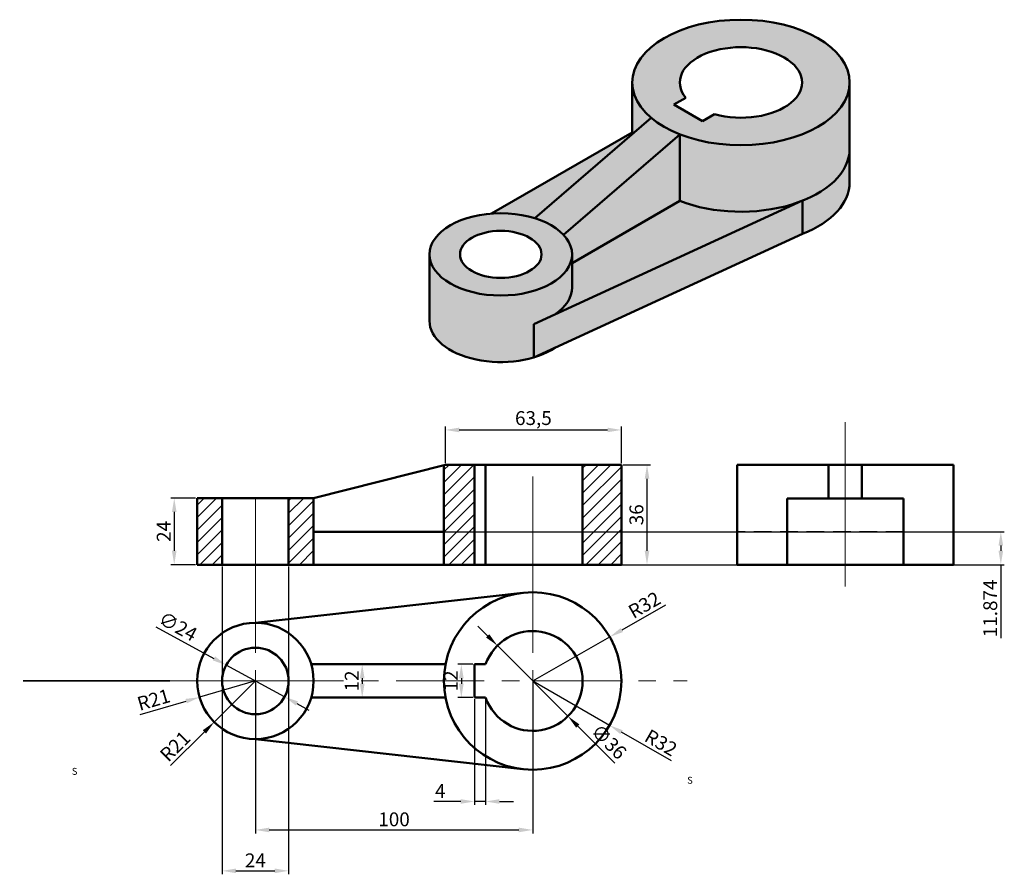
# Model space of a CAD drawing. Units: millimetres. Extents: x -12 to 343, y -126 to 182.
import ezdxf

# ---------------------------------------------------------------- set-up
doc = ezdxf.new("R2010")
doc.units = ezdxf.units.MM
for name, pattern in [('CENTER', [50.800000000000004, 31.75, -6.349999999999999, 6.349999999999999, -6.349999999999999]), ('HIDDEN', [9.524999999999999, 6.349999999999999, -3.174999999999999]), ('PHANTOM', [63.50000000000001, 31.75, -6.349999999999999, 6.349999999999999, -6.349999999999999, 6.349999999999999, -6.349999999999999])]:
    doc.linetypes.add(name, pattern=pattern)
for name, color, linetype, lineweight in [('M-CNTR', 1, 'CENTER', 18), ('M-DIMS', 2, 'Continuous', 25), ('M-HATC', 251, 'Continuous', 18), ('M-HIDN', 4, 'HIDDEN', 25), ('M-OUTL', 7, 'Continuous', 50), ('M-SECT', 6, 'PHANTOM', 35), ('M-TEXT', 3, 'Continuous', 25)]:
    doc.layers.add(name, color=color, linetype=linetype, lineweight=lineweight)
doc.styles.get("Standard").update_dxf_attribs({"font": 'arial.ttf'})
doc.dimstyles.new('ISO-25', dxfattribs={"dimtxt": 5, "dimasz": 5, "dimexe": 1.25, "dimexo": 0.625, "dimtad": 1, "dimtxsty": 'Standard', "dimcen": 5, "dimadec": 0, "dimazin": 0, "dimtfac": 1, "dimtmove": 0, "dimatfit": 3, "dimfxl": 1, "dimarcsym": 0})
pattern_1 = [(45, (0, 0), (-2.245064030267288, 2.245064030267288), [])]

# ---------------------------------------------------------------- blocks, each defined once
blk = doc.blocks.new('*D1')
at = {"layer": 'Defpoints', "color": 0, "transparency": 16777216}
for p in [(205.2649197556575, 34.47405386195669), (141.7649197556575, 21.88545579629272), (205.2649197556575, 21.88545579629272)]:
    blk.add_point(p, dxfattribs=at)
at = {"layer": 'M-DIMS', "color": 0, "lineweight": -2, "transparency": 16777216}
for p, q in [((141.7649197556575, 22.51045579629272), (141.7649197556575, 35.72405386195669)), ((205.2649197556575, 22.51045579629272), (205.2649197556575, 35.72405386195669)), ((146.7649197556575, 34.47405386195669), (200.2649197556575, 34.47405386195669))]:
    blk.add_line(p, q, dxfattribs=at)
at = {"layer": 'M-DIMS', "color": 0, "transparency": 16777216}
for points in [[(146.7649197556575, 35.30738719529003), (146.7649197556575, 33.64072052862336), (141.7649197556575, 34.47405386195669)], [(200.2649197556575, 35.30738719529003), (200.2649197556575, 33.64072052862336), (205.2649197556575, 34.47405386195669)]]:
    blk.add_solid(points, dxfattribs=at)
at = {"layer": 'M-DIMS', "color": 0, "transparency": 16777216, "insert": (173.5149197556575, 38.10382875963745), "char_height": 5, "attachment_point": 5}
blk.add_mtext('63,5', dxfattribs=at)
blk = doc.blocks.new('*D2')
at = {"layer": 'Defpoints', "color": 0, "transparency": 16777216}
for p in [(205.2649197556577, 21.88545579629272), (214.4923014426937, 21.88545579629272), (205.2649197556577, -14.11454420370729)]:
    blk.add_point(p, dxfattribs=at)
at = {"layer": 'M-DIMS', "color": 0, "lineweight": -2, "transparency": 16777216}
for p, q in [((205.8899197556577, 21.88545579629272), (215.7423014426937, 21.88545579629272)), ((214.4923014426937, -9.114544203707284), (214.4923014426937, 16.88545579629272)), ((205.8899197556577, -14.11454420370729), (215.7423014426937, -14.11454420370728))]:
    blk.add_line(p, q, dxfattribs=at)
at = {"layer": 'M-DIMS', "color": 0, "transparency": 16777216}
for points in [[(213.6589681093604, 16.88545579629272), (215.3256347760271, 16.88545579629272), (214.4923014426937, 21.88545579629272)], [(213.6589681093604, -9.114544203707284), (215.3256347760271, -9.114544203707284), (214.4923014426937, -14.11454420370728)]]:
    blk.add_solid(points, dxfattribs=at)
at = {"layer": 'M-DIMS', "color": 0, "transparency": 16777216, "insert": (211.3127311834849, 3.885455796292659), "char_height": 5, "attachment_point": 5, "rotation": 90}
blk.add_mtext('36', dxfattribs=at)
blk = doc.blocks.new('*D3')
at = {"layer": 'Defpoints', "color": 0, "transparency": 16777216}
for p in [(52.26491975565753, 9.88545579629272), (43.9988590508993, -14.11454420370729), (52.26491975565753, -14.11454420370729)]:
    blk.add_point(p, dxfattribs=at)
at = {"layer": 'M-DIMS', "color": 0, "lineweight": -2, "transparency": 16777216}
for p, q in [((51.63991975565753, 9.88545579629272), (42.7488590508993, 9.885455796292717)), ((43.9988590508993, 4.885455796292717), (43.9988590508993, -9.114544203707291)), ((51.63991975565753, -14.11454420370729), (42.7488590508993, -14.11454420370729))]:
    blk.add_line(p, q, dxfattribs=at)
at = {"layer": 'M-DIMS', "color": 0, "transparency": 16777216}
for points in [[(43.16552571756596, 4.885455796292717), (44.83219238423263, 4.885455796292717), (43.9988590508993, 9.885455796292717)], [(43.16552571756596, -9.114544203707291), (44.83219238423263, -9.11454420370729), (43.9988590508993, -14.11454420370729)]]:
    blk.add_solid(points, dxfattribs=at)
at = {"layer": 'M-DIMS', "color": 0, "transparency": 16777216, "insert": (40.86362712729765, -2.114544203707298), "char_height": 5, "attachment_point": 5, "rotation": 90}
blk.add_mtext('24', dxfattribs=at)
blk = doc.blocks.new('*D4')
at = {"layer": 'Defpoints', "color": 0, "transparency": 16777216}
for p in [(73.2649197556575, -56.05038137719969), (53.10428194249988, -61.92819414783812)]:
    blk.add_point(p, dxfattribs=at)
at = {"layer": 'M-DIMS', "color": 0, "lineweight": -2, "transparency": 16777216}
for p, q in [((73.2649197556575, -56.05038137719969), (53.10428194249988, -61.92819414783812)), ((31.76063262380506, -68.15091267986675), (48.30413008222426, -63.3276733789425))]:
    blk.add_line(p, q, dxfattribs=at)
at = {"layer": 'M-DIMS', "color": 0, "transparency": 16777216}
blk.add_solid([(48.07088354370687, -62.52764806889658), (48.53737662074166, -64.12769868898843), (53.10428194249988, -61.92819414783812)], dxfattribs=at)
at = {"layer": 'M-DIMS', "color": 0, "transparency": 16777216, "insert": (36.75476703052166, -63.42911477486243), "char_height": 5, "attachment_point": 5, "rotation": 16.253988585853655}
blk.add_mtext('R21', dxfattribs=at)
blk = doc.blocks.new('*D5')
at = {"layer": 'Defpoints', "color": 0, "transparency": 16777216}
for p in [(201.0521765959829, -40.18002040809157), (173.2649197556575, -56.05038137719977)]:
    blk.add_point(p, dxfattribs=at)
at = {"layer": 'M-DIMS', "color": 0, "lineweight": -2, "transparency": 16777216}
for p, q in [((221.1513216491535, -28.70063296811324), (205.3939354772837, -37.70027650666842)), ((173.2649197556575, -56.05038137719977), (201.0521765959829, -40.18002040809157))]:
    blk.add_line(p, q, dxfattribs=at)
at = {"layer": 'M-DIMS', "color": 0, "transparency": 16777216}
blk.add_solid([(204.9806448270465, -36.97665002645161), (205.8072261275209, -38.42390298688524), (201.0521765959829, -40.18002040809157)], dxfattribs=at)
at = {"layer": 'M-DIMS', "color": 0, "transparency": 16777216, "insert": (213.8666040119852, -29.19959730435135), "char_height": 5, "attachment_point": 5, "rotation": 29.732333460001456}
blk.add_mtext('R32', dxfattribs=at)
blk = doc.blocks.new('*D6')
at = {"layer": 'Defpoints', "color": 0, "transparency": 16777216}
for p in [(62.72135419654524, -50.32035299151955), (83.8084853147698, -61.78040976287999)]:
    blk.add_point(p, dxfattribs=at)
at = {"layer": 'M-DIMS', "color": 0, "lineweight": -2, "transparency": 16777216}
for p, q in [((37.38314425713691, -36.54999595422157), (58.32820188024844, -47.93284116415278)), ((83.8084853147698, -61.78040976287999), (62.72135419654524, -50.32035299151955)), ((88.20163763106659, -64.16792159024676), (92.59478994736337, -66.55543341761353))]:
    blk.add_line(p, q, dxfattribs=at)
at = {"layer": 'M-DIMS', "color": 0, "transparency": 16777216}
for points in [[(58.7261205181429, -47.20064911143665), (57.93028324235399, -48.66503321686892), (62.72135419654524, -50.32035299151955)], [(88.59955626896105, -63.43572953753064), (87.80371899317213, -64.90011364296289), (83.8084853147698, -61.78040976287999)]]:
    blk.add_solid(points, dxfattribs=at)
at = {"layer": 'M-DIMS', "color": 0, "transparency": 16777216, "insert": (45.04389919536463, -36.93733442097821), "char_height": 5, "attachment_point": 5, "rotation": 331.47759577174867}
blk.add_mtext('∅24', dxfattribs=at)
blk = doc.blocks.new('*D7')
at = {"layer": 'Defpoints', "color": 0, "transparency": 16777216}
for p in [(117.6109920089049, -50.05038137719978), (111.7946377354413, -62.05038137719979), (117.6109920089049, -62.05038137719978)]:
    blk.add_point(p, dxfattribs=at)
at = {"layer": 'M-DIMS', "color": 0, "lineweight": -2, "transparency": 16777216}
for p, q in [((116.9859920089049, -50.05038137719978), (110.5446377354413, -50.05038137719979)), ((111.7946377354413, -55.05038137719979), (111.7946377354413, -57.05038137719979)), ((116.9859920089049, -62.05038137719978), (110.5446377354413, -62.05038137719979))]:
    blk.add_line(p, q, dxfattribs=at)
at = {"layer": 'M-DIMS', "color": 0, "transparency": 16777216}
for points in [[(110.961304402108, -55.05038137719979), (112.6279710687746, -55.05038137719978), (111.7946377354413, -50.05038137719979)], [(110.961304402108, -57.05038137719979), (112.6279710687746, -57.05038137719978), (111.7946377354413, -62.05038137719979)]]:
    blk.add_solid(points, dxfattribs=at)
at = {"layer": 'M-DIMS', "color": 0, "transparency": 16777216, "insert": (108.6594058118396, -56.0503813771998), "char_height": 5, "attachment_point": 5, "rotation": 90}
blk.add_mtext('12', dxfattribs=at)
blk = doc.blocks.new('*D8')
at = {"layer": 'Defpoints', "color": 0, "transparency": 16777216}
for p in [(73.2649197556575, -56.0503813771997), (173.2649197556575, -56.05038137719976), (173.2649197556575, -109.7895127931604)]:
    blk.add_point(p, dxfattribs=at)
at = {"layer": 'M-DIMS', "color": 0, "lineweight": -2, "transparency": 16777216}
for p, q in [((73.2649197556575, -56.6753813771997), (73.2649197556575, -111.0395127931603)), ((173.2649197556575, -56.67538137719976), (173.2649197556575, -111.0395127931603)), ((78.2649197556575, -109.7895127931604), (168.2649197556575, -109.7895127931604))]:
    blk.add_line(p, q, dxfattribs=at)
at = {"layer": 'M-DIMS', "color": 0, "transparency": 16777216}
for points in [[(78.2649197556575, -108.956179459827), (78.2649197556575, -110.6228461264937), (73.2649197556575, -109.7895127931604)], [(168.2649197556575, -108.956179459827), (168.2649197556575, -110.6228461264937), (173.2649197556575, -109.7895127931604)]]:
    blk.add_solid(points, dxfattribs=at)
at = {"layer": 'M-DIMS', "color": 0, "transparency": 16777216, "insert": (123.2649197556575, -106.6116478545519), "char_height": 5, "attachment_point": 5}
blk.add_mtext('100', dxfattribs=at)
blk = doc.blocks.new('*D9')
at = {"layer": 'Defpoints', "color": 0, "transparency": 16777216}
for p in [(152.2943570071803, -62.05038137719975), (156.2943570071803, -62.05038137719975), (152.2943570071803, -99.52431760050536)]:
    blk.add_point(p, dxfattribs=at)
at = {"layer": 'M-DIMS', "color": 0, "lineweight": -2, "transparency": 16777216}
for p, q in [((152.2943570071803, -62.67538137719975), (152.2943570071803, -100.7743176005053)), ((156.2943570071803, -62.67538137719975), (156.2943570071803, -100.7743176005053)), ((147.2943570071803, -99.52431760050536), (137.585966829827, -99.52431760050536)), ((156.2943570071803, -99.52431760050536), (152.2943570071803, -99.52431760050536)), ((161.2943570071803, -99.52431760050536), (166.2943570071803, -99.52431760050536))]:
    blk.add_line(p, q, dxfattribs=at)
at = {"layer": 'M-DIMS', "color": 0, "transparency": 16777216}
for points in [[(147.2943570071803, -98.69098426717203), (147.2943570071803, -100.3576509338387), (152.2943570071803, -99.52431760050536)], [(161.2943570071803, -98.69098426717203), (161.2943570071803, -100.3576509338387), (156.2943570071803, -99.52431760050536)]]:
    blk.add_solid(points, dxfattribs=at)
at = {"layer": 'M-DIMS', "color": 0, "transparency": 16777216, "insert": (139.9401619185037, -96.39931760050536), "char_height": 5, "attachment_point": 5}
blk.add_mtext('4', dxfattribs=at)
blk = doc.blocks.new('*D10')
at = {"layer": 'Defpoints', "color": 0, "transparency": 16777216}
for p in [(152.2943570071803, -50.05038137719978), (147.5338658392859, -62.05038137719978), (152.2943570071804, -62.05038137719978)]:
    blk.add_point(p, dxfattribs=at)
at = {"layer": 'M-DIMS', "color": 0, "lineweight": -2, "transparency": 16777216}
for p, q in [((151.6693570071803, -50.05038137719978), (146.2838658392859, -50.05038137719978)), ((147.5338658392859, -55.05038137719978), (147.5338658392859, -57.05038137719978)), ((151.6693570071804, -62.05038137719978), (146.2838658392859, -62.05038137719978))]:
    blk.add_line(p, q, dxfattribs=at)
at = {"layer": 'M-DIMS', "color": 0, "transparency": 16777216}
for points in [[(146.7005325059526, -55.05038137719978), (148.3671991726193, -55.05038137719978), (147.5338658392859, -50.05038137719978)], [(146.7005325059526, -57.05038137719978), (148.3671991726193, -57.05038137719978), (147.5338658392859, -62.05038137719978)]]:
    blk.add_solid(points, dxfattribs=at)
at = {"layer": 'M-DIMS', "color": 0, "transparency": 16777216, "insert": (144.3986339156843, -56.05038137719981), "char_height": 5, "attachment_point": 5, "rotation": 90}
blk.add_mtext('12', dxfattribs=at)
blk = doc.blocks.new('*D11')
at = {"layer": 'Defpoints', "color": 0, "transparency": 16777216}
for p in [(94.26492000000003, -2.24086), (94.26492000000003, -14.11454400000001), (342.0873210000002, -14.11454399999997)]:
    blk.add_point(p, dxfattribs=at)
at = {"layer": 'M-DIMS', "color": 0, "lineweight": -2, "transparency": 16777216}
for p, q in [((94.88992000000003, -2.24086), (343.3373210000002, -2.24085999999996)), ((342.0873210000002, -7.240859999999962), (342.0873210000002, -9.114543999999967)), ((94.88992000000003, -14.11454400000001), (343.3373210000002, -14.11454399999997)), ((342.0873210000002, -14.11454399999997), (342.0873210000002, -40.63057401364254))]:
    blk.add_line(p, q, dxfattribs=at)
at = {"layer": 'M-DIMS', "color": 0, "transparency": 16777216}
for points in [[(341.2539876666669, -7.240859999999963), (342.9206543333335, -7.240859999999962), (342.0873210000002, -2.24085999999996)], [(341.2539876666669, -9.114543999999967), (342.9206543333335, -9.114543999999967), (342.0873210000002, -14.11454399999997)]]:
    blk.add_solid(points, dxfattribs=at)
at = {"layer": 'M-DIMS', "color": 0, "transparency": 16777216, "insert": (338.9094560613917, -29.87255900682135), "char_height": 5, "attachment_point": 5, "rotation": 90}
blk.add_mtext('11.874', dxfattribs=at)
blk = doc.blocks.new('*D12')
at = {"layer": 'Defpoints', "color": 0, "transparency": 16777216}
for p in [(61.26491999999999, -14.114544), (85.26492, -14.114544), (85.26492, -124.541948)]:
    blk.add_point(p, dxfattribs=at)
at = {"layer": 'M-DIMS', "color": 0, "lineweight": -2, "transparency": 16777216}
for p, q in [((61.26491999999999, -14.739544), (61.26491999999998, -125.791948)), ((85.26492, -14.739544), (85.26492, -125.791948)), ((66.26491999999998, -124.541948), (80.26492, -124.541948))]:
    blk.add_line(p, q, dxfattribs=at)
at = {"layer": 'M-DIMS', "color": 0, "transparency": 16777216}
for points in [[(66.26491999999998, -123.7086146666666), (66.26491999999998, -125.3752813333333), (61.26491999999998, -124.541948)], [(80.26492, -123.7086146666666), (80.26492, -125.3752813333333), (85.26492, -124.541948)]]:
    blk.add_solid(points, dxfattribs=at)
at = {"layer": 'M-DIMS', "color": 0, "transparency": 16777216, "insert": (73.26491999999999, -121.4067160763983), "char_height": 5, "attachment_point": 5}
blk.add_mtext('24', dxfattribs=at)
blk = doc.blocks.new('*D13')
at = {"layer": 'Defpoints', "color": 0, "transparency": 16777216}
for p in [(173.2649199999999, -56.05038099999997), (200.983459, -72.040458)]:
    blk.add_point(p, dxfattribs=at)
at = {"layer": 'M-DIMS', "color": 0, "lineweight": -2, "transparency": 16777216}
for p, q in [((173.2649199999999, -56.05038099999997), (200.983459, -72.040458)), ((223.3082809938933, -84.91904524060625), (205.3144807890435, -74.53890757180046))]:
    blk.add_line(p, q, dxfattribs=at)
at = {"layer": 'M-DIMS', "color": 0, "transparency": 16777216}
blk.add_solid([(205.7308890510103, -73.81707060695987), (204.8980725270769, -75.26074453664106), (200.983459, -72.040458)], dxfattribs=at)
at = {"layer": 'M-DIMS', "color": 0, "transparency": 16777216, "insert": (219.2033818604532, -78.88034674122817), "char_height": 5, "attachment_point": 5, "rotation": 330.0205129811975}
blk.add_mtext('R32', dxfattribs=at)
blk = doc.blocks.new('*D14')
at = {"layer": 'Defpoints', "color": 0, "transparency": 16777216}
for p in [(73.26492, -56.050381), (58.40803300000002, -70.89197500000003)]:
    blk.add_point(p, dxfattribs=at)
at = {"layer": 'M-DIMS', "color": 0, "lineweight": -2, "transparency": 16777216}
for p, q in [((73.26492, -56.050381), (58.40803300000002, -70.89197500000003)), ((42.67935478698478, -86.60446283101184), (54.87067896758761, -74.42568784195191))]:
    blk.add_line(p, q, dxfattribs=at)
at = {"layer": 'M-DIMS', "color": 0, "transparency": 16777216}
blk.add_solid([(54.28172682726231, -73.83612883654985), (55.45963110791291, -75.01524684735398), (58.40803300000002, -70.89197500000003)], dxfattribs=at)
at = {"layer": 'M-DIMS', "color": 0, "transparency": 16777216, "insert": (44.79053799889427, -80.06384669995774), "char_height": 5, "attachment_point": 5, "rotation": 44.97049599005939}
blk.add_mtext('R21', dxfattribs=at)
blk = doc.blocks.new('*D15')
at = {"layer": 'Defpoints', "color": 0, "transparency": 16777216}
for p in [(160.5442609999999, -43.31519999999999), (185.985579, -68.78556199999997)]:
    blk.add_point(p, dxfattribs=at)
at = {"layer": 'M-DIMS', "color": 0, "lineweight": -2, "transparency": 16777216}
for p, q in [((157.0107446138214, -39.77764972493566), (153.4772282276428, -36.24009944987133)), ((160.5442609999999, -43.31519999999999), (185.985579, -68.78556199999997)), ((202.8396808624512, -85.65890463191496), (189.5190953861785, -72.32311227506428))]:
    blk.add_line(p, q, dxfattribs=at)
at = {"layer": 'M-DIMS', "color": 0, "transparency": 16777216}
for points in [[(157.6003363263321, -39.18873032723924), (156.4211529013107, -40.36656912263207), (160.5442609999999, -43.31519999999999)], [(190.1086870986892, -71.73419287736787), (188.9295036736678, -72.91203167276072), (185.985579, -68.78556199999997)]]:
    blk.add_solid(points, dxfattribs=at)
at = {"layer": 'M-DIMS', "color": 0, "transparency": 16777216, "insert": (200.293453295623, -78.4151532604248), "char_height": 5, "attachment_point": 5, "rotation": 314.96731401439416}
blk.add_mtext('∅36', dxfattribs=at)

msp = doc.modelspace()

# ---------------------------------------------------------------- hatches: boundary and pattern name
at = {"layer": 'M-HATC'}
h = msp.add_hatch(color=256, dxfattribs=at)
h.dxf.hatch_style = 1
edge = h.paths.add_edge_path()
edge.add_ellipse((248.360351945901, 159.8042998001659), major_axis=(-39.19183588453085, 0), ratio=0.5773502691896261, start_angle=40.3567508759614, end_angle=180)
edge.add_ellipse((248.360351945901, 159.8042998001659), major_axis=(-39.19183588453085, 0), ratio=0.5773502691896261, start_angle=180, end_angle=360)
edge.add_ellipse((248.360351945901, 159.8042998001659), major_axis=(-39.19183588453085, 0), ratio=0.5773502691896261, start_angle=0, end_angle=21.41833269324282)
edge.add_ellipse((248.360351945901, 159.8042998001659), major_axis=(-39.19183588453085, 0), ratio=0.5773502691896261, start_angle=21.41833269324282, end_angle=40.3567508759614)
edge = h.paths.add_edge_path(flags=16)
edge.add_ellipse((248.360351945901, 159.8042998001659), major_axis=(-22.0454076850486, 0), ratio=0.5773502691896253, start_angle=50.401969701232076, end_angle=375.4155559432115, ccw=False)
edge.add_line((238.8595659119086, 148.3190184259274), (234.50394548535, 145.8042998001659))
edge.add_line((234.50394548535, 145.8042998001659), (224.1116406399367, 151.8042998001659))
edge.add_line((224.1116406399367, 151.8042998001659), (228.4672610664953, 154.3190184259273))
edge = h.paths.add_edge_path()
edge.add_line((173.6876422966888, 72.64908361327036), (181.2815148595527, 76.1377766444114))
edge.add_ellipse((161.7578115674571, 85.80429980016594), major_axis=(-25.71964229922337, 0), ratio=0.5773502691896261, start_angle=153.6591923730604, end_angle=180)
edge.add_line((187.4774538666805, 85.80429980016616), (187.4774538666805, 97.80429980016592))
edge.add_ellipse((161.7578115674571, 97.80429980016595), major_axis=(-25.71964229922337, 0), ratio=0.5773502691896261, start_angle=0, end_angle=180, ccw=False)
edge.add_line((136.0381692682337, 97.804299800166), (136.0381692682337, 73.80429980016598))
edge.add_ellipse((161.7578115674571, 73.80429980016595), major_axis=(-25.71964229922337, 0), ratio=0.5773502691896261, start_angle=0, end_angle=132.2033678326249)
edge.add_line((173.6876422966888, 60.64908361327036), (173.6876422966888, 72.64908361327036))
h.paths.add_polyline_path([(270.6214639644938, 105.1813489804948), (270.6214639644938, 117.1813489804948), (173.6876422966888, 72.64908361327036), (173.6876422966888, 60.64908361327036)])
edge = h.paths.add_edge_path()
edge.add_ellipse((248.360351945901, 135.8042998001659), major_axis=(-39.19183588453085, 0), ratio=0.5773502691896261, start_angle=40.35675087596138, end_angle=140.0852005292437, ccw=False)
edge.add_line((226.3351891909752, 117.0880661546642), (187.4774538666805, 94.65354220508348))
edge.add_line((187.4774538666805, 94.65354220508348), (187.4774538666805, 85.80429980016615))
edge.add_ellipse((161.7578115674571, 85.80429980016594), major_axis=(-25.71964229922337, 0), ratio=0.5773502691896261, start_angle=153.6591923730604, end_angle=180, ccw=False)
edge.add_line((181.2815148595527, 76.1377766444114), (270.6214639644939, 117.1813489804949))
edge = h.paths.add_edge_path()
edge.add_line((226.3351891909752, 117.0880661546642), (226.3351891909752, 141.0880661546642))
edge.add_line((226.3351891909752, 141.0880661546642), (184.3823890480971, 104.866605698915))
edge.add_ellipse((161.7578115674571, 97.80429980016595), major_axis=(-25.71964229922337, 0), ratio=0.5773502691896261, start_angle=180, end_angle=197.3358550375143, ccw=False)
edge.add_line((187.4774538666805, 97.80429980016595), (187.4774538666805, 94.65354220508348))
edge.add_line((187.4774538666805, 94.65354220508348), (226.3351891909752, 117.0880661546642))
edge = h.paths.add_edge_path()
edge.add_ellipse((248.360351945901, 159.8042998001659), major_axis=(-39.19183588453085, 0), ratio=0.5773502691896261, start_angle=21.418332693242803, end_angle=40.35675087596138, ccw=False)
edge.add_line((215.942884345562, 147.0880661546642), (173.9900842026838, 110.866605698915))
edge.add_ellipse((161.7578115674571, 97.80429980016595), major_axis=(-25.71964229922337, 0), ratio=0.5773502691896261, start_angle=197.3358550375143, end_angle=226.8794677220288, ccw=False)
edge.add_line((184.3823890480971, 104.866605698915), (226.3351891909752, 141.0880661546642))
edge = h.paths.add_edge_path()
edge.add_line((209.1685160613701, 141.2391713947708), (209.1685160613701, 141.8042998001659))
edge.add_line((209.1685160613701, 141.8042998001659), (158.4664551590954, 112.5314512897688))
edge.add_ellipse((161.7578115674571, 97.80429980016595), major_axis=(-25.71964229922337, 0), ratio=0.5773502691896261, start_angle=226.8794677220288, end_angle=282.597954751084, ccw=False)
edge.add_line((173.9900842026838, 110.866605698915), (209.1685160613701, 141.2391713947708))
edge = h.paths.add_edge_path()
edge.add_ellipse((161.7578115674571, 97.80429980016595), major_axis=(-25.71964229922337, 0), ratio=0.5773502691896261, start_angle=197.3358550375143, end_angle=226.8794677220287)
edge.add_ellipse((161.7578115674571, 97.80429980016595), major_axis=(-25.71964229922337, 0), ratio=0.5773502691896261, start_angle=226.8794677220287, end_angle=282.597954751084)
edge.add_ellipse((161.7578115674571, 97.80429980016595), major_axis=(-25.71964229922337, 0), ratio=0.5773502691896261, start_angle=282.597954751084, end_angle=360)
edge.add_ellipse((161.7578115674571, 97.80429980016595), major_axis=(-25.71964229922337, 0), ratio=0.5773502691896261, start_angle=0, end_angle=180)
edge.add_ellipse((161.7578115674571, 97.80429980016595), major_axis=(-25.71964229922337, 0), ratio=0.5773502691896261, start_angle=180, end_angle=197.3358550375143)
edge = h.paths.add_edge_path(flags=16)
edge.add_ellipse((161.7578115674571, 97.80429980016595), major_axis=(-14.69693845669906, 0), ratio=0.5773502691896257, start_angle=0, end_angle=360)
edge = h.paths.add_edge_path()
edge.add_ellipse((248.360351945901, 135.8042998001659), major_axis=(-39.19183588453085, 0), ratio=0.5773502691896261, start_angle=140.0852005292436, end_angle=180)
edge.add_line((287.5521878304318, 135.8042998001659), (287.5521878304318, 159.8042998001659))
edge.add_ellipse((248.360351945901, 159.8042998001659), major_axis=(-39.19183588453085, 0), ratio=0.5773502691896261, start_angle=40.35675087596138, end_angle=180, ccw=False)
edge.add_line((226.3351891909752, 141.0880661546642), (226.3351891909752, 117.0880661546642))
edge.add_ellipse((248.360351945901, 135.8042998001659), major_axis=(-39.19183588453085, 0), ratio=0.5773502691896261, start_angle=40.35675087596138, end_angle=140.0852005292436)
h = msp.add_hatch(color=256, dxfattribs=at)
h.dxf.hatch_style = 1
edge = h.paths.add_edge_path()
edge.add_ellipse((248.360351945901, 159.8042998001659), major_axis=(-39.19183588453085, 0), ratio=0.5773502691896261, start_angle=0, end_angle=21.418332693242803, ccw=False)
edge.add_line((209.1685160613701, 159.8042998001659), (209.1685160613701, 141.2391713947708))
edge.add_line((209.1685160613701, 141.2391713947708), (215.942884345562, 147.0880661546642))
h = msp.add_hatch(color=256, dxfattribs=at)
h.dxf.hatch_style = 1
edge = h.paths.add_edge_path()
edge.add_ellipse((248.360351945901, 123.8042998001659), major_axis=(-39.19183588453085, 0), ratio=0.5773502691896261, start_angle=140.0852005292436, end_angle=180)
edge.add_line((287.5521878304318, 123.8042998001659), (287.5521878304318, 135.8042998001659))
edge.add_ellipse((248.360351945901, 135.8042998001659), major_axis=(-39.19183588453085, 0), ratio=0.5773502691896261, start_angle=140.0852005292437, end_angle=180, ccw=False)
edge.add_line((270.6214639644938, 117.1813489804948), (270.6214639644938, 105.1813489804948))
h = msp.add_hatch(color=256, dxfattribs=at)
h.dxf.hatch_style = 1
edge = h.paths.add_edge_path()
edge.add_ellipse((161.7578115674571, 97.80429980016595), major_axis=(-25.71964229922337, 0), ratio=0.5773502691896261, start_angle=171.8101999361156, end_angle=180, ccw=False)
edge.add_line((186.7137658331746, 94.21262671336197), (187.4774538666805, 94.65354220508348))
edge.add_line((187.4774538666805, 94.65354220508348), (187.4774538666805, 97.80429980016596))
h = msp.add_hatch(dxfattribs=at)
h.set_pattern_fill('ANSI31', color=256)
h.set_pattern_definition(pattern_1)
h.paths.add_polyline_path([(152.2943570071803, 21.88545579629272), (141.7649197556575, 21.88545579629272), (141.2649197556575, 21.75914000681903), (141.2649197556575, -2.240859993180976), (141.2649197556575, -14.11454420370728), (152.2943570071803, -14.11454420370728)])
h = msp.add_hatch(dxfattribs=at)
h.set_pattern_fill('ANSI31', color=256)
h.set_pattern_definition(pattern_1)
h.paths.add_polyline_path([(205.2649197556575, 21.88545579629272), (191.2649197556575, 21.88545579629272), (191.2649197556575, -14.11454420370728), (205.2649197556575, -14.11454420370728)])
h = msp.add_hatch(dxfattribs=at)
h.set_pattern_fill('ANSI31', color=256)
h.set_pattern_definition(pattern_1)
h.paths.add_polyline_path([(61.2649197556575, 9.885455796292717), (52.2649197556575, 9.885455796292717), (52.2649197556575, -14.11454420370728), (61.2649197556575, -14.11454420370728)])
h.paths.add_polyline_path([(94.26491975565752, 9.885455796292717), (85.2649197556575, 9.885455796292717), (85.2649197556575, -14.11454420370728), (94.26491975565752, -14.11454420370728)])

# ---------------------------------------------------------------- linework, layer by layer
at = {"layer": 'M-CNTR'}
for p, q in [((285.9873205459853, 9.759140006819022), (285.9873205459853, 37.26564665224896)), ((173.2649197556575, -14.11454420370728), (173.2649197556575, 21.88545579629272)), ((73.26491975565747, -14.11454420370728), (73.2649197556575, 9.885455796292717)), ((285.9873205459853, 9.759140006819022), (285.9873205459853, -26.53155776970061)), ((73.26491975565747, -14.11454420370728), (73.26491975565747, -107.4419484592936)), ((173.2649197556575, -14.11454420370728), (173.2649197556575, -104.9242523515736)), ((73.2649197556575, -56.05038137719976), (42.3913057095624, -56.05038137719976)), ((73.2649197556575, -56.05038137719976), (173.2649197556575, -56.05038137719976)), ((173.2649197556575, -56.05038137719976), (228.9815345269417, -56.05038137719976))]:
    msp.add_line(p, q, dxfattribs=at)
at = {"layer": 'M-HIDN'}
for q in [(246.9873205459853, -2.240859993181119), (324.9873205459853, -2.240859993180976)]:
    msp.add_line((306.9873205459853, -2.240859993180976), q, dxfattribs=at)
at = {"layer": 'M-OUTL'}
for p, q in [((209.1685160613701, 159.8042998001659), (209.1685160613701, 141.2391713947708)), ((287.5521878304318, 159.8042998001659), (287.5521878304318, 123.8042998001659)), ((224.1116406399367, 151.8042998001659), (228.4672610664953, 154.3190184259273)), ((224.1116406399367, 151.8042998001659), (234.50394548535, 145.8042998001659)), ((173.9900842026838, 110.866605698915), (215.942884345562, 147.0880661546642)), ((234.50394548535, 145.8042998001659), (238.8595659119086, 148.3190184259274)), ((209.1685160613701, 141.8042998001659), (158.4664551590954, 112.5314512897688)), ((184.3823890480971, 104.866605698915), (226.3351891909752, 141.0880661546642)), ((226.3351891909752, 141.0880661546642), (226.3351891909752, 117.0880661546642)), ((173.6876422966888, 72.64908361327036), (270.6214639644938, 117.1813489804948)), ((270.6214639644938, 117.1813489804949), (270.6214639644938, 105.1813489804948)), ((226.3351891909752, 117.0880661546642), (187.4774538666805, 94.6535422050835)), ((173.6876422966888, 60.64908361327035), (270.6214639644938, 105.1813489804948)), ((136.0381692682337, 97.80429980016595), (136.0381692682337, 73.80429980016595)), ((187.4774538666805, 97.80429980016595), (187.4774538666805, 85.80429980016596)), ((173.6876422966888, 72.64908361327036), (173.6876422966888, 60.64908361327035)), ((94.26491975565752, 9.885455796292717), (141.7649197556575, 21.88545579629272)), ((141.2649197556575, 21.75914000681903), (141.2649197556575, -2.240859993180976)), ((141.2649197556575, -14.11454420370728), (141.2649197556575, 21.75914000681903)), ((205.2649197556575, 21.88545579629272), (141.7649197556575, 21.88545579629272)), ((152.2943570071803, 21.88545579629272), (156.2943570071803, 21.88545579629272)), ((152.2943570071803, -14.11454420370728), (152.2943570071803, 21.88545579629272)), ((156.2943570071803, 21.88545579629272), (156.2943570071803, -14.11454420370728)), ((191.2649197556575, -14.11454420370728), (191.2649197556575, 21.88545579629272)), ((205.2649197556575, -14.11454420370728), (205.2649197556575, 21.88545579629272)), ((205.2649197556575, -14.11454420370728), (205.2649197556575, 21.88545579629272)), ((246.9873205459853, 21.88545579629272), (324.9873205459853, 21.88545579629272)), ((246.9873205459853, -2.240859993180976), (246.9873205459853, 21.88545579629272)), ((279.9873205459853, 9.759140006819022), (279.9873205459854, 21.88545579629272)), ((291.9873205459853, 9.759140006819022), (291.9873205459853, 21.88545579629272)), ((324.9873205459853, -2.240859993180976), (324.9873205459853, 21.88545579629272)), ((52.26491975565751, -14.11454420370728), (52.2649197556575, 9.885455796292717)), ((52.2649197556575, -14.11454420370728), (52.2649197556575, 9.885455796292717)), ((52.2649197556575, 9.885455796292717), (94.26491975565752, 9.885455796292717)), ((61.2649197556575, -14.11454420370728), (61.2649197556575, 9.885455796292717)), ((85.26491975565749, -14.11454420370728), (85.2649197556575, 9.885455796292717)), ((94.26491975565752, -2.240859993180976), (94.26491975565752, 9.885455796292717)), ((94.26491975565749, -14.11454420370728), (94.26491975565752, 9.885455796292717)), ((264.9873205459853, -2.240859993180976), (264.9873205459853, 9.759140006819022)), ((264.9873205459853, 9.759140006819022), (306.9873205459853, 9.759140006819022)), ((306.9873205459853, 9.759140006819022), (306.9873205459853, -2.240859993180976)), ((141.2649197556575, -2.240859993180976), (94.26491975565752, -2.240859993180976)), ((246.9873205459853, -14.11454420370728), (246.9873205459853, -2.240859993180976)), ((264.9873205459853, -2.240859993180976), (264.9873205459853, -14.11454420370728)), ((306.9873205459853, -2.240859993180976), (306.9873205459853, -14.11454420370728)), ((324.9873205459853, -2.240859993180976), (324.9873205459853, -14.11454420370728)), ((52.2649197556575, -14.11454420370728), (205.2649197556575, -14.11454420370728)), ((324.9873205459853, -14.11454420370728), (246.9873205459854, -14.11454420370728)), ((73.2649197556575, -35.05038137719976), (169.70316374113, -24.24921954161618)), ((93.3895315531556, -50.05038137719975), (141.8324524646541, -50.05038137719975)), ((156.2943570071803, -50.05038137719975), (152.2943570071803, -50.05038137719975)), ((152.2943570071803, -50.05038137719975), (152.2943570071803, -62.05038137719975)), ((152.2943570071803, -50.05038137719975), (156.2943570071803, -50.05038137719974)), ((152.2943570071803, -56.05038137719976), (152.2943570071803, -50.05038137719975)), ((93.3895315531556, -62.05038137719976), (141.8324524646541, -62.05038137719975)), ((152.2943570071803, -62.05038137719976), (156.2943570071803, -62.05038137719975)), ((73.2649197556575, -77.05038137719976), (169.70316374113, -87.85154321278333))]:
    msp.add_line(p, q, dxfattribs=at)
for centre, radius in [((173.2649197556575, -56.05038137719976), 32), ((73.2649197556575, -56.05038137719976), 21), ((73.2649197556575, -56.05038137719976), 12)]:
    msp.add_circle(centre, radius, dxfattribs=at)
msp.add_arc((173.2649197556575, -56.05038137719976), 18, 199.4712206344907, 160.5287793655093, dxfattribs=at)
for centre, major_axis, ratio in [((248.360351945901, 159.8042998001659), (-39.19183588453085, 0), 0.5773502691896261), ((161.7578115674571, 97.80429980016595), (-25.71964229922337, 0), 0.5773502691896261), ((161.7578115674571, 97.80429980016595), (-14.69693845669906, 0), 0.5773502691896257)]:
    msp.add_ellipse(centre, major_axis=major_axis, ratio=ratio, dxfattribs=at)
for centre, major_axis, ratio, start_param, end_param in [((248.360351945901, 159.8042998001659), (-22.0454076850486, 0), 0.5773502691896253, 1.12523507285157, 6.728746561122913), ((248.360351945901, 135.8042998001659), (-39.19183588453085, 0), 0.5773502691896261, 0.9740145495728517, 3.141592653589793), ((248.360351945901, 123.8042998001659), (-39.19183588453085, 0), 0.5773502691896261, 2.174874715790936, 3.141592653589793), ((161.7578115674571, 85.80429980016594), (-25.71964229922337, 0), 0.5773502691896261, 2.432721171922723, 3.141592653589793), ((161.7578115674571, 73.80429980016595), (-25.71964229922337, 0), 0.5773502691896261, 0, 2.432721171923374)]:
    msp.add_ellipse(centre, major_axis=major_axis, ratio=ratio, start_param=start_param, end_param=end_param, dxfattribs=at)
at = {"layer": 'M-SECT'}
for p, q in [((21.29615275860033, -56.05038137719976), (-11.73054822914219, -56.05038137719976)), ((42.3913057095624, -56.05038137719976), (21.29615275860033, -56.05038137719976))]:
    msp.add_line(p, q, dxfattribs=at)
for points in [[(4.78280226472907, -56.05038137719976, 0, 10, 0), (4.78280226472907, -76.4786706528605, 0, 0, 0), (4.78280226472907, -87.4055129809874, 0, 0, 0)], [(228.9815345269417, -56.05038137719976, 0, 10, 0), (228.9815345269417, -76.4786706528605, 0, 0, 0), (228.9815345269417, -87.4055129809874, 0, 0, 0)]]:
    msp.add_lwpolyline(points, format="xyseb", dxfattribs=at)

# ---------------------------------------------------------------- texts
at = {"layer": 'M-TEXT', "char_height": 2.5, "attachment_point": 1}
for width, insert in [(6.728317833870278, (7.052337335846459, -87.4055129809874)), (7.133775386088927, (228.9815345269417, -90.63121798525093))]:
    msp.add_mtext_dynamic_manual_height_columns('S', width=width, gutter_width=12.5, heights=[0], dxfattribs=dict(at, insert=insert))

# ---------------------------------------------------------------- dimensions: what is measured, and where the dimension line sits
at = {"layer": 'M-DIMS'}
for base, p1, p2, override, picture, middle in [((205.2649197556575, 34.47405386195669), (141.7649197556575, 21.88545579629272), (205.2649197556575, 21.88545579629272), {"dimclrd": 0, "dimclre": 0, "dimclrt": 0}, '*D1', (173.5149197556575, 38.10382875963745)), ((85.26492, -124.541948), (61.26491999999999, -14.114544), (85.26492, -14.114544), {"dimdec": 0, "dimlfac": 1, "dimrnd": 0, "dimzin": 0, "dimdsep": 46, "dimlunit": 2}, '*D12', (73.26491999999999, -121.4067160763983)), ((173.2649197556575, -109.7895127931604), (73.2649197556575, -56.0503813771997), (173.2649197556575, -56.05038137719976), {"dimclrd": 0, "dimclre": 0, "dimclrt": 0}, '*D8', (123.2649197556575, -106.6116478545519)), ((152.2943570071803, -99.52431760050536), (156.2943570071803, -62.05038137719975), (152.2943570071803, -62.05038137719975), {"dimclrd": 0, "dimclre": 0, "dimclrt": 0}, '*D9', (139.9401619185037, -96.39931760050536))]:
    dim = msp.add_linear_dim(base=base, p1=p1, p2=p2, dimstyle='ISO-25', override=override, dxfattribs=at)
    dim.commit()
    dim.dimension.update_dxf_attribs({"geometry": picture, "text_midpoint": middle})
for base, p1, p2, override, picture, middle in [((214.4923014426937, 21.88545579629272), (205.2649197556575, -14.11454420370728), (205.2649197556575, 21.88545579629272), {"dimclrd": 0, "dimclre": 0, "dimclrt": 0}, '*D2', (211.3127311834849, 3.885455796292659)), ((43.9988590508993, -14.11454420370729), (52.2649197556575, 9.885455796292717), (52.2649197556575, -14.11454420370728), {"dimclrd": 0, "dimclre": 0, "dimclrt": 0}, '*D3', (40.86362712729765, -2.114544203707298)), ((342.0873210000002, -14.11454399999997), (94.26492, -2.24086), (94.26492, -14.114544), {"dimdec": 3, "dimlfac": 1, "dimrnd": 0, "dimzin": 0, "dimdsep": 46, "dimlunit": 2}, '*D11', (338.9094560613917, -29.87255900682135)), ((111.7946377354413, -62.05038137719979), (117.6109920089049, -50.05038137719975), (117.6109920089048, -62.05038137719975), {"dimclrd": 0, "dimclre": 0, "dimclrt": 0}, '*D7', (108.6594058118396, -56.0503813771998)), ((147.5338658392859, -62.05038137719978), (152.2943570071802, -50.05038137719975), (152.2943570071803, -62.05038137719975), {"dimclrd": 0, "dimclre": 0, "dimclrt": 0}, '*D10', (144.3986339156843, -56.05038137719981))]:
    dim = msp.add_linear_dim(base=base, p1=p1, p2=p2, angle=90, dimstyle='ISO-25', override=override, dxfattribs=at)
    dim.commit()
    dim.dimension.update_dxf_attribs({"geometry": picture, "text_midpoint": middle})
for center, mpoint, override, picture, middle in [((173.2649197556575, -56.05038137719977), (201.0521765959829, -40.18002040809157), {"dimclrd": 0, "dimclre": 0, "dimclrt": 0}, '*D5', (213.8666040119852, -29.19959730435135)), ((73.2649197556575, -56.05038137719969), (53.10428194249988, -61.92819414783812), {"dimclrd": 0, "dimclre": 0, "dimclrt": 0}, '*D4', (36.75476703052166, -63.42911477486243)), ((73.26492, -56.050381), (58.40803300000002, -70.89197500000003), {"dimdec": 0, "dimlfac": 1, "dimrnd": 0, "dimzin": 0, "dimdsep": 46, "dimlunit": 2}, '*D14', (44.79053799889427, -80.06384669995774))]:
    dim = msp.add_radius_dim(center=center, mpoint=mpoint, dimstyle='ISO-25', override=override, dxfattribs=at)
    dim.commit()
    dim.dimension.update_dxf_attribs({"geometry": picture, "text_midpoint": middle})
for p1, p2, override, picture, middle in [((83.8084853147698, -61.78040976287999), (62.72135419654524, -50.32035299151955), {"dimclrd": 0, "dimclre": 0, "dimclrt": 0}, '*D6', (43.45968901114156, -39.85236778774336)), ((160.5442609999999, -43.31519999999999), (185.985579, -68.78556199999997), {"dimdec": 0, "dimlfac": 1, "dimrnd": 0, "dimzin": 0, "dimdsep": 46, "dimlunit": 2}, '*D15', (197.9461463174042, -80.7597835910218))]:
    dim = msp.add_diameter_dim_2p(p1=p1, p2=p2, dimstyle='ISO-25', override=override, dxfattribs=at)
    dim.commit()
    dim.dimension.update_dxf_attribs({"geometry": picture, "text_midpoint": middle, "dimtype": 163})
dim = msp.add_radius_dim(center=(173.2649199999999, -56.05038099999997), mpoint=(200.983459, -72.040458), dimstyle='ISO-25', override={"dimdec": 0, "dimlfac": 1, "dimrnd": 0, "dimzin": 0, "dimdsep": 46, "dimlunit": 2}, dxfattribs=at)
dim.commit()
dim.dimension.update_dxf_attribs({"geometry": '*D13', "text_midpoint": (217.6145826699273, -81.63450435571374), "dimtype": 164})

doc.saveas('drawing.dxf')
